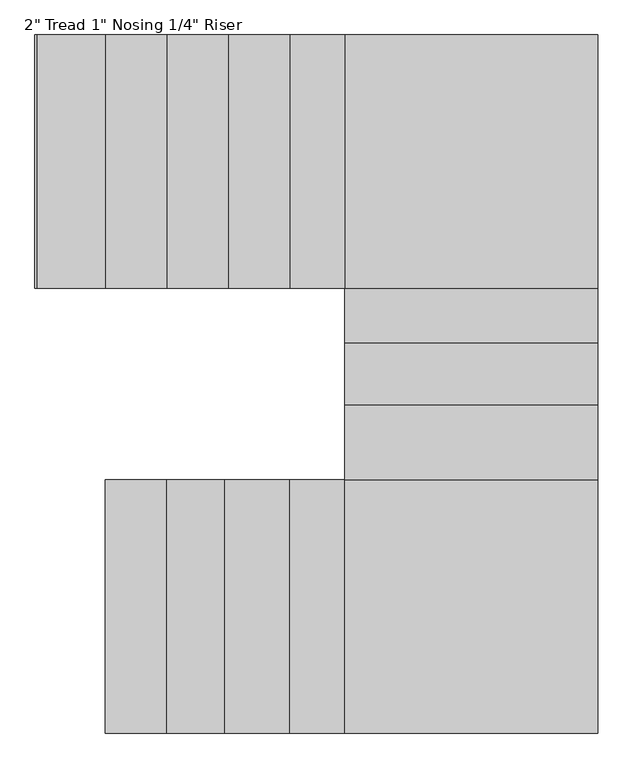
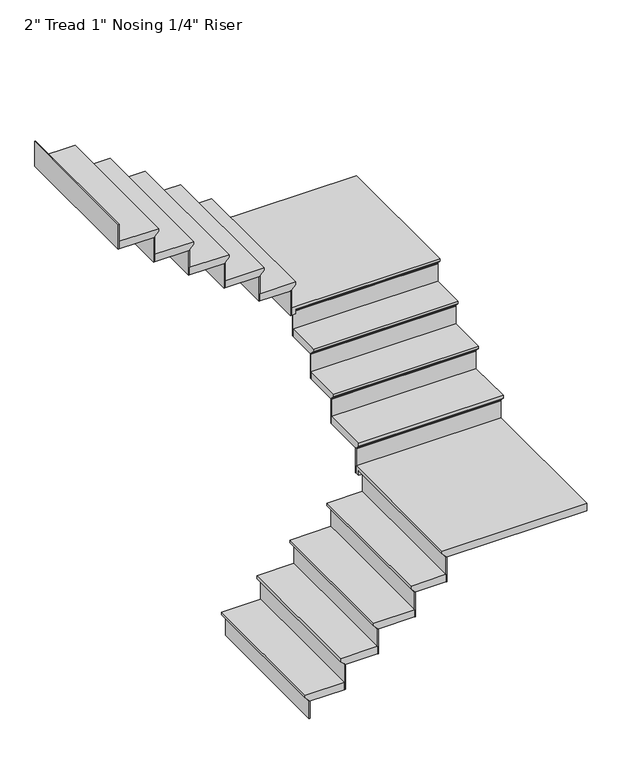
"""IFC4 building model written with IfcOpenShell, lengths in millimetres: stair flight geometry."""

from ifc_helpers import new_model, si_unit, origin, place, context, project, spatial, faceted_brep, source, transform, mapped, element, save


def stair_flight_3d22c4e0(model_context):
    return source(origin(), model_context, "Body", "Brep", [
        faceted_brep([(344.764115, -6141.1350571, 150.2833333), (344.764115, -6141.1350571, 169.3333333), (344.764115, -5201.3350571, 169.3333333), (344.764115, -5201.3350571, 150.2833333), (370.164115, -6141.1350571, 124.8833333), (370.164115, -5201.3350571, 124.8833333), (598.764115, -6141.1350571, 169.3333333), (598.764115, -5201.3350571, 169.3333333), (370.164115, -5201.3350571, 118.5333333), (598.764115, -5201.3350571, 118.5333333), (598.764115, -6141.1350571, 118.5333333), (370.164115, -6141.1350571, 118.5333333)], [[[0, 1, 2, 3]], [[4, 0, 3, 5]], [[2, 1, 6, 7]], [[8, 9, 10, 11]], [[2, 7, 9, 8, 5, 3]], [[8, 11, 4, 5]], [[6, 1, 0, 4, 11, 10]], [[7, 6, 10, 9]]]),
        faceted_brep([(370.164115, -6141.1350571, 118.5333333), (370.164115, -6141.1350571, 0.0), (376.514115, -6141.1350571, 0.0), (376.514115, -6141.1350571, 118.5333333), (370.164115, -5201.3350571, 118.5333333), (376.514115, -5201.3350571, 118.5333333), (376.514115, -5201.3350571, 0.0), (370.164115, -5201.3350571, 0.0)], [[[0, 1, 2, 3]], [[4, 5, 6, 7]], [[1, 0, 4, 7]], [[2, 1, 7, 6]], [[3, 2, 6, 5]], [[0, 3, 5, 4]]]),
        faceted_brep([(598.764115, -6141.1350571, 287.8666667), (598.764115, -6141.1350571, 118.5333333), (605.114115, -6141.1350571, 118.5333333), (605.114115, -6141.1350571, 287.8666667), (598.764115, -5201.3350571, 287.8666667), (605.114115, -5201.3350571, 287.8666667), (605.114115, -5201.3350571, 118.5333333), (598.764115, -5201.3350571, 118.5333333)], [[[0, 1, 2, 3]], [[4, 5, 6, 7]], [[1, 0, 4, 7]], [[2, 1, 7, 6]], [[3, 2, 6, 5]], [[0, 3, 5, 4]]]),
        faceted_brep([(573.364115, -5201.3350571, 338.6666667), (573.364115, -6141.1350571, 338.6666667), (814.664115, -6141.1350571, 338.6666667), (814.664115, -5201.3350571, 338.6666667), (598.764115, -5201.3350571, 287.8666667), (814.664115, -5201.3350571, 287.8666667), (814.664115, -6141.1350571, 287.8666667), (598.764115, -6141.1350571, 287.8666667), (598.764115, -5201.3350571, 294.2166667), (573.364115, -5201.3350571, 319.6166667), (598.764115, -6141.1350571, 294.2166667), (573.364115, -6141.1350571, 319.6166667)], [[[0, 1, 2, 3]], [[4, 5, 6, 7]], [[0, 3, 5, 4, 8, 9]], [[4, 7, 10, 8]], [[2, 1, 11, 10, 7, 6]], [[3, 2, 6, 5]], [[11, 1, 0, 9]], [[10, 11, 9, 8]]]),
        faceted_brep([(814.664115, -6141.1350571, 457.2), (814.664115, -6141.1350571, 287.8666667), (821.014115, -6141.1350571, 287.8666667), (821.014115, -6141.1350571, 457.2), (814.664115, -5201.3350571, 457.2), (821.014115, -5201.3350571, 457.2), (821.014115, -5201.3350571, 287.8666667), (814.664115, -5201.3350571, 287.8666667)], [[[0, 1, 2, 3]], [[4, 5, 6, 7]], [[1, 0, 4, 7]], [[2, 1, 7, 6]], [[3, 2, 6, 5]], [[0, 3, 5, 4]]]),
        faceted_brep([(789.264115, -5201.3350571, 508.0), (789.264115, -6141.1350571, 508.0), (1055.964115, -6141.1350571, 508.0), (1055.964115, -5201.3350571, 508.0), (814.664115, -5201.3350571, 457.2), (1055.964115, -5201.3350571, 457.2), (1055.964115, -6141.1350571, 457.2), (814.664115, -6141.1350571, 457.2), (814.664115, -5201.3350571, 463.55), (789.264115, -5201.3350571, 488.95), (814.664115, -6141.1350571, 463.55), (789.264115, -6141.1350571, 488.95)], [[[0, 1, 2, 3]], [[4, 5, 6, 7]], [[0, 3, 5, 4, 8, 9]], [[4, 7, 10, 8]], [[2, 1, 11, 10, 7, 6]], [[3, 2, 6, 5]], [[11, 1, 0, 9]], [[10, 11, 9, 8]]]),
        faceted_brep([(1055.964115, -6141.1350571, 626.5333333), (1055.964115, -6141.1350571, 457.2), (1062.314115, -6141.1350571, 457.2), (1062.314115, -6141.1350571, 626.5333333), (1055.964115, -5201.3350571, 626.5333333), (1062.314115, -5201.3350571, 626.5333333), (1062.314115, -5201.3350571, 457.2), (1055.964115, -5201.3350571, 457.2)], [[[0, 1, 2, 3]], [[4, 5, 6, 7]], [[1, 0, 4, 7]], [[2, 1, 7, 6]], [[3, 2, 6, 5]], [[0, 3, 5, 4]]]),
        faceted_brep([(1030.564115, -5201.3350571, 677.3333333), (1030.564115, -6141.1350571, 677.3333333), (1259.164115, -6141.1350571, 677.3333333), (1259.164115, -5201.3350571, 677.3333333), (1055.964115, -5201.3350571, 626.5333333), (1259.164115, -5201.3350571, 626.5333333), (1259.164115, -6141.1350571, 626.5333333), (1055.964115, -6141.1350571, 626.5333333), (1055.964115, -5201.3350571, 632.8833333), (1030.564115, -5201.3350571, 658.2833333), (1055.964115, -6141.1350571, 632.8833333), (1030.564115, -6141.1350571, 658.2833333)], [[[0, 1, 2, 3]], [[4, 5, 6, 7]], [[0, 3, 5, 4, 8, 9]], [[4, 7, 10, 8]], [[2, 1, 11, 10, 7, 6]], [[3, 2, 6, 5]], [[11, 1, 0, 9]], [[10, 11, 9, 8]]]),
        faceted_brep([(1259.164115, -6141.1350571, 795.8666667), (1259.164115, -6141.1350571, 626.5333333), (1265.514115, -6141.1350571, 626.5333333), (1265.514115, -6141.1350571, 795.8666667), (1259.164115, -5201.3350571, 795.8666667), (1265.514115, -5201.3350571, 795.8666667), (1265.514115, -5201.3350571, 626.5333333), (1259.164115, -5201.3350571, 626.5333333)], [[[0, 1, 2, 3]], [[4, 5, 6, 7]], [[1, 0, 4, 7]], [[2, 1, 7, 6]], [[3, 2, 6, 5]], [[0, 3, 5, 4]]]),
        faceted_brep([(2173.564115, -6141.1350571, 846.6666667), (2173.564115, -5175.9350571, 846.6666667), (1233.764115, -5175.9350571, 846.6666667), (1233.764115, -6141.1350571, 846.6666667), (1233.764115, -5201.3350571, 795.8666667), (1233.764115, -5175.9350571, 795.8666667), (2173.564115, -5175.9350571, 795.8666667), (2173.564115, -6141.1350571, 795.8666667), (1259.164115, -6141.1350571, 795.8666667), (1259.164115, -5201.3350571, 795.8666667), (1233.764115, -5201.3350571, 827.6166667), (1233.764115, -6141.1350571, 827.6166667), (1259.164115, -5201.3350571, 802.2166667), (1259.164115, -6141.1350571, 802.2166667)], [[[0, 1, 2, 3]], [[4, 5, 6, 7, 8, 9]], [[3, 2, 5, 4, 10, 11]], [[4, 9, 12, 10]], [[9, 8, 13, 12]], [[0, 3, 11, 13, 8, 7]], [[1, 0, 7, 6]], [[2, 1, 6, 5]], [[13, 11, 10, 12]]]),
        faceted_brep([(2173.564115, -5175.9350571, 965.2), (2173.564115, -5175.9350571, 795.8666667), (2173.564115, -5169.5850571, 795.8666667), (2173.564115, -5169.5850571, 965.2), (1233.764115, -5175.9350571, 965.2), (1233.764115, -5169.5850571, 965.2), (1233.764115, -5169.5850571, 795.8666667), (1233.764115, -5175.9350571, 795.8666667)], [[[0, 1, 2, 3]], [[4, 5, 6, 7]], [[1, 0, 4, 7]], [[2, 1, 7, 6]], [[3, 2, 6, 5]], [[0, 3, 5, 4]]]),
        faceted_brep([(1233.764115, -5201.3350571, 1016.0), (2173.564115, -5201.3350571, 1016.0), (2173.564115, -4896.5350571, 1016.0), (1233.764115, -4896.5350571, 1016.0), (1233.764115, -5175.9350571, 965.2), (1233.764115, -4896.5350571, 965.2), (2173.564115, -4896.5350571, 965.2), (2173.564115, -5175.9350571, 965.2), (1233.764115, -5175.9350571, 971.55), (1233.764115, -5201.3350571, 996.95), (2173.564115, -5175.9350571, 971.55), (2173.564115, -5201.3350571, 996.95)], [[[0, 1, 2, 3]], [[4, 5, 6, 7]], [[0, 3, 5, 4, 8, 9]], [[4, 7, 10, 8]], [[2, 1, 11, 10, 7, 6]], [[3, 2, 6, 5]], [[11, 1, 0, 9]], [[10, 11, 9, 8]]]),
        faceted_brep([(2173.564115, -4896.5350571, 1134.5333333), (2173.564115, -4896.5350571, 965.2), (2173.564115, -4890.1850571, 965.2), (2173.564115, -4890.1850571, 1134.5333333), (1233.764115, -4896.5350571, 1134.5333333), (1233.764115, -4890.1850571, 1134.5333333), (1233.764115, -4890.1850571, 965.2), (1233.764115, -4896.5350571, 965.2)], [[[0, 1, 2, 3]], [[4, 5, 6, 7]], [[1, 0, 4, 7]], [[2, 1, 7, 6]], [[3, 2, 6, 5]], [[0, 3, 5, 4]]]),
        faceted_brep([(1233.764115, -4921.9350571, 1185.3333333), (2173.564115, -4921.9350571, 1185.3333333), (2173.564115, -4667.9350571, 1185.3333333), (1233.764115, -4667.9350571, 1185.3333333), (1233.764115, -4896.5350571, 1134.5333333), (1233.764115, -4667.9350571, 1134.5333333), (2173.564115, -4667.9350571, 1134.5333333), (2173.564115, -4896.5350571, 1134.5333333), (1233.764115, -4896.5350571, 1140.8833333), (1233.764115, -4921.9350571, 1166.2833333), (2173.564115, -4896.5350571, 1140.8833333), (2173.564115, -4921.9350571, 1166.2833333)], [[[0, 1, 2, 3]], [[4, 5, 6, 7]], [[0, 3, 5, 4, 8, 9]], [[4, 7, 10, 8]], [[2, 1, 11, 10, 7, 6]], [[3, 2, 6, 5]], [[11, 1, 0, 9]], [[10, 11, 9, 8]]]),
        faceted_brep([(2173.564115, -4667.9350571, 1303.8666667), (2173.564115, -4667.9350571, 1134.5333333), (2173.564115, -4661.5850571, 1134.5333333), (2173.564115, -4661.5850571, 1303.8666667), (1233.764115, -4667.9350571, 1303.8666667), (1233.764115, -4661.5850571, 1303.8666667), (1233.764115, -4661.5850571, 1134.5333333), (1233.764115, -4667.9350571, 1134.5333333)], [[[0, 1, 2, 3]], [[4, 5, 6, 7]], [[1, 0, 4, 7]], [[2, 1, 7, 6]], [[3, 2, 6, 5]], [[0, 3, 5, 4]]]),
        faceted_brep([(1233.764115, -4693.3350571, 1354.6666667), (2173.564115, -4693.3350571, 1354.6666667), (2173.564115, -4464.7350571, 1354.6666667), (1233.764115, -4464.7350571, 1354.6666667), (1233.764115, -4667.9350571, 1303.8666667), (1233.764115, -4464.7350571, 1303.8666667), (2173.564115, -4464.7350571, 1303.8666667), (2173.564115, -4667.9350571, 1303.8666667), (1233.764115, -4667.9350571, 1310.2166667), (1233.764115, -4693.3350571, 1335.6166667), (2173.564115, -4667.9350571, 1310.2166667), (2173.564115, -4693.3350571, 1335.6166667)], [[[0, 1, 2, 3]], [[4, 5, 6, 7]], [[0, 3, 5, 4, 8, 9]], [[4, 7, 10, 8]], [[2, 1, 11, 10, 7, 6]], [[3, 2, 6, 5]], [[11, 1, 0, 9]], [[10, 11, 9, 8]]]),
        faceted_brep([(2173.564115, -4464.7350571, 1473.2), (2173.564115, -4464.7350571, 1303.8666667), (2173.564115, -4458.3850571, 1303.8666667), (2173.564115, -4458.3850571, 1473.2), (1233.764115, -4464.7350571, 1473.2), (1233.764115, -4458.3850571, 1473.2), (1233.764115, -4458.3850571, 1303.8666667), (1233.764115, -4464.7350571, 1303.8666667)], [[[0, 1, 2, 3]], [[4, 5, 6, 7]], [[1, 0, 4, 7]], [[2, 1, 7, 6]], [[3, 2, 6, 5]], [[0, 3, 5, 4]]]),
        faceted_brep([(2173.564115, -3550.3350571, 1524.0), (1208.364115, -3550.3350571, 1524.0), (1208.364115, -4490.1350571, 1524.0), (2173.564115, -4490.1350571, 1524.0), (1233.764115, -4490.1350571, 1473.2), (1208.364115, -4490.1350571, 1473.2), (1208.364115, -3550.3350571, 1473.2), (2173.564115, -3550.3350571, 1473.2), (2173.564115, -4464.7350571, 1473.2), (1233.764115, -4464.7350571, 1473.2), (1233.764115, -4490.1350571, 1504.95), (2173.564115, -4490.1350571, 1504.95), (1233.764115, -4464.7350571, 1479.55), (2173.564115, -4464.7350571, 1479.55)], [[[0, 1, 2, 3]], [[4, 5, 6, 7, 8, 9]], [[3, 2, 5, 4, 10, 11]], [[4, 9, 12, 10]], [[9, 8, 13, 12]], [[0, 3, 11, 13, 8, 7]], [[1, 0, 7, 6]], [[2, 1, 6, 5]], [[13, 11, 10, 12]]]),
        faceted_brep([(1208.364115, -3550.3350571, 1642.5333333), (1208.364115, -3550.3350571, 1473.2), (1202.014115, -3550.3350571, 1473.2), (1202.014115, -3550.3350571, 1642.5333333), (1208.364115, -4490.1350571, 1642.5333333), (1202.014115, -4490.1350571, 1642.5333333), (1202.014115, -4490.1350571, 1473.2), (1208.364115, -4490.1350571, 1473.2)], [[[0, 1, 2, 3]], [[4, 5, 6, 7]], [[1, 0, 4, 7]], [[2, 1, 7, 6]], [[3, 2, 6, 5]], [[0, 3, 5, 4]]]),
        faceted_brep([(1233.764115, -4490.1350571, 1693.3333333), (1233.764115, -3550.3350571, 1693.3333333), (1005.164115, -3550.3350571, 1693.3333333), (1005.164115, -4490.1350571, 1693.3333333), (1208.364115, -4490.1350571, 1642.5333333), (1005.164115, -4490.1350571, 1642.5333333), (1005.164115, -3550.3350571, 1642.5333333), (1208.364115, -3550.3350571, 1642.5333333), (1208.364115, -4490.1350571, 1648.8833333), (1233.764115, -4490.1350571, 1674.2833333), (1208.364115, -3550.3350571, 1648.8833333), (1233.764115, -3550.3350571, 1674.2833333)], [[[0, 1, 2, 3]], [[4, 5, 6, 7]], [[0, 3, 5, 4, 8, 9]], [[4, 7, 10, 8]], [[2, 1, 11, 10, 7, 6]], [[3, 2, 6, 5]], [[11, 1, 0, 9]], [[10, 11, 9, 8]]]),
        faceted_brep([(1005.164115, -3550.3350571, 1811.8666667), (1005.164115, -3550.3350571, 1642.5333333), (998.814115, -3550.3350571, 1642.5333333), (998.814115, -3550.3350571, 1811.8666667), (1005.164115, -4490.1350571, 1811.8666667), (998.814115, -4490.1350571, 1811.8666667), (998.814115, -4490.1350571, 1642.5333333), (1005.164115, -4490.1350571, 1642.5333333)], [[[0, 1, 2, 3]], [[4, 5, 6, 7]], [[1, 0, 4, 7]], [[2, 1, 7, 6]], [[3, 2, 6, 5]], [[0, 3, 5, 4]]]),
        faceted_brep([(1030.564115, -4490.1350571, 1862.6666667), (1030.564115, -3550.3350571, 1862.6666667), (776.564115, -3550.3350571, 1862.6666667), (776.564115, -4490.1350571, 1862.6666667), (1005.164115, -4490.1350571, 1811.8666667), (776.564115, -4490.1350571, 1811.8666667), (776.564115, -3550.3350571, 1811.8666667), (1005.164115, -3550.3350571, 1811.8666667), (1005.164115, -4490.1350571, 1818.2166667), (1030.564115, -4490.1350571, 1843.6166667), (1005.164115, -3550.3350571, 1818.2166667), (1030.564115, -3550.3350571, 1843.6166667)], [[[0, 1, 2, 3]], [[4, 5, 6, 7]], [[0, 3, 5, 4, 8, 9]], [[4, 7, 10, 8]], [[2, 1, 11, 10, 7, 6]], [[3, 2, 6, 5]], [[11, 1, 0, 9]], [[10, 11, 9, 8]]]),
        faceted_brep([(776.564115, -3550.3350571, 1981.2), (776.564115, -3550.3350571, 1811.8666667), (770.214115, -3550.3350571, 1811.8666667), (770.214115, -3550.3350571, 1981.2), (776.564115, -4490.1350571, 1981.2), (770.214115, -4490.1350571, 1981.2), (770.214115, -4490.1350571, 1811.8666667), (776.564115, -4490.1350571, 1811.8666667)], [[[0, 1, 2, 3]], [[4, 5, 6, 7]], [[1, 0, 4, 7]], [[2, 1, 7, 6]], [[3, 2, 6, 5]], [[0, 3, 5, 4]]]),
        faceted_brep([(801.964115, -4490.1350571, 2032.0), (801.964115, -3550.3350571, 2032.0), (547.964115, -3550.3350571, 2032.0), (547.964115, -4490.1350571, 2032.0), (776.564115, -4490.1350571, 1981.2), (547.964115, -4490.1350571, 1981.2), (547.964115, -3550.3350571, 1981.2), (776.564115, -3550.3350571, 1981.2), (776.564115, -4490.1350571, 1987.55), (801.964115, -4490.1350571, 2012.95), (776.564115, -3550.3350571, 1987.55), (801.964115, -3550.3350571, 2012.95)], [[[0, 1, 2, 3]], [[4, 5, 6, 7]], [[0, 3, 5, 4, 8, 9]], [[4, 7, 10, 8]], [[2, 1, 11, 10, 7, 6]], [[3, 2, 6, 5]], [[11, 1, 0, 9]], [[10, 11, 9, 8]]]),
        faceted_brep([(547.964115, -3550.3350571, 2150.5333333), (547.964115, -3550.3350571, 1981.2), (541.614115, -3550.3350571, 1981.2), (541.614115, -3550.3350571, 2150.5333333), (547.964115, -4490.1350571, 2150.5333333), (541.614115, -4490.1350571, 2150.5333333), (541.614115, -4490.1350571, 1981.2), (547.964115, -4490.1350571, 1981.2)], [[[0, 1, 2, 3]], [[4, 5, 6, 7]], [[1, 0, 4, 7]], [[2, 1, 7, 6]], [[3, 2, 6, 5]], [[0, 3, 5, 4]]]),
        faceted_brep([(573.364115, -4490.1350571, 2201.3333333), (573.364115, -3550.3350571, 2201.3333333), (319.364115, -3550.3350571, 2201.3333333), (319.364115, -4490.1350571, 2201.3333333), (547.964115, -4490.1350571, 2150.5333333), (319.364115, -4490.1350571, 2150.5333333), (319.364115, -3550.3350571, 2150.5333333), (547.964115, -3550.3350571, 2150.5333333), (547.964115, -4490.1350571, 2156.8833333), (573.364115, -4490.1350571, 2182.2833333), (547.964115, -3550.3350571, 2156.8833333), (573.364115, -3550.3350571, 2182.2833333)], [[[0, 1, 2, 3]], [[4, 5, 6, 7]], [[0, 3, 5, 4, 8, 9]], [[4, 7, 10, 8]], [[2, 1, 11, 10, 7, 6]], [[3, 2, 6, 5]], [[11, 1, 0, 9]], [[10, 11, 9, 8]]]),
        faceted_brep([(319.364115, -3550.3350571, 2319.8666667), (319.364115, -3550.3350571, 2150.5333333), (313.014115, -3550.3350571, 2150.5333333), (313.014115, -3550.3350571, 2319.8666667), (319.364115, -4490.1350571, 2319.8666667), (313.014115, -4490.1350571, 2319.8666667), (313.014115, -4490.1350571, 2150.5333333), (319.364115, -4490.1350571, 2150.5333333)], [[[0, 1, 2, 3]], [[4, 5, 6, 7]], [[1, 0, 4, 7]], [[2, 1, 7, 6]], [[3, 2, 6, 5]], [[0, 3, 5, 4]]]),
        faceted_brep([(90.764115, -3550.3350571, 2489.2), (90.764115, -3550.3350571, 2319.8666667), (84.414115, -3550.3350571, 2319.8666667), (84.414115, -3550.3350571, 2489.2), (90.764115, -4490.1350571, 2489.2), (84.414115, -4490.1350571, 2489.2), (84.414115, -4490.1350571, 2319.8666667), (90.764115, -4490.1350571, 2319.8666667)], [[[0, 1, 2, 3]], [[4, 5, 6, 7]], [[1, 0, 4, 7]], [[2, 1, 7, 6]], [[3, 2, 6, 5]], [[0, 3, 5, 4]]]),
        faceted_brep([(344.764115, -4490.1350571, 2370.6666667), (344.764115, -3550.3350571, 2370.6666667), (90.764115, -3550.3350571, 2370.6666667), (90.764115, -4490.1350571, 2370.6666667), (319.364115, -4490.1350571, 2319.8666667), (90.764115, -4490.1350571, 2319.8666667), (90.764115, -3550.3350571, 2319.8666667), (319.364115, -3550.3350571, 2319.8666667), (319.364115, -4490.1350571, 2326.2166667), (344.764115, -4490.1350571, 2351.6166667), (319.364115, -3550.3350571, 2326.2166667), (344.764115, -3550.3350571, 2351.6166667)], [[[0, 1, 2, 3]], [[4, 5, 6, 7]], [[0, 3, 5, 4, 8, 9]], [[4, 7, 10, 8]], [[2, 1, 11, 10, 7, 6]], [[3, 2, 6, 5]], [[11, 1, 0, 9]], [[10, 11, 9, 8]]]),
    ])


if __name__ == "__main__":
    model = new_model("IFC4")
    model_context = context("Model", 3, world=origin())
    ifc_project = project(units=[si_unit("LENGTHUNIT", "METRE", prefix="MILLI")], contexts=[model_context])
    site = spatial("IfcSite", under=ifc_project)
    building = spatial("IfcBuilding", under=site)
    placement = place(None, origin())
    stair_flight_shape = stair_flight_3d22c4e0(model_context)
    element("IfcStairFlight", 1, ObjectType="2\" Tread 1\" Nosing 1/4\" Riser", at=placement, inside=building, context=model_context, shape_type="MappedRepresentation", body=[
        mapped(stair_flight_shape, transform((0.0, 0.0, 0.0), x_axis=(1.0, 0.0, 0.0), y_axis=(0.0, 1.0, 0.0), z_axis=(0.0, 0.0, 1.0))),
    ])
    save(model, "model.ifc")
